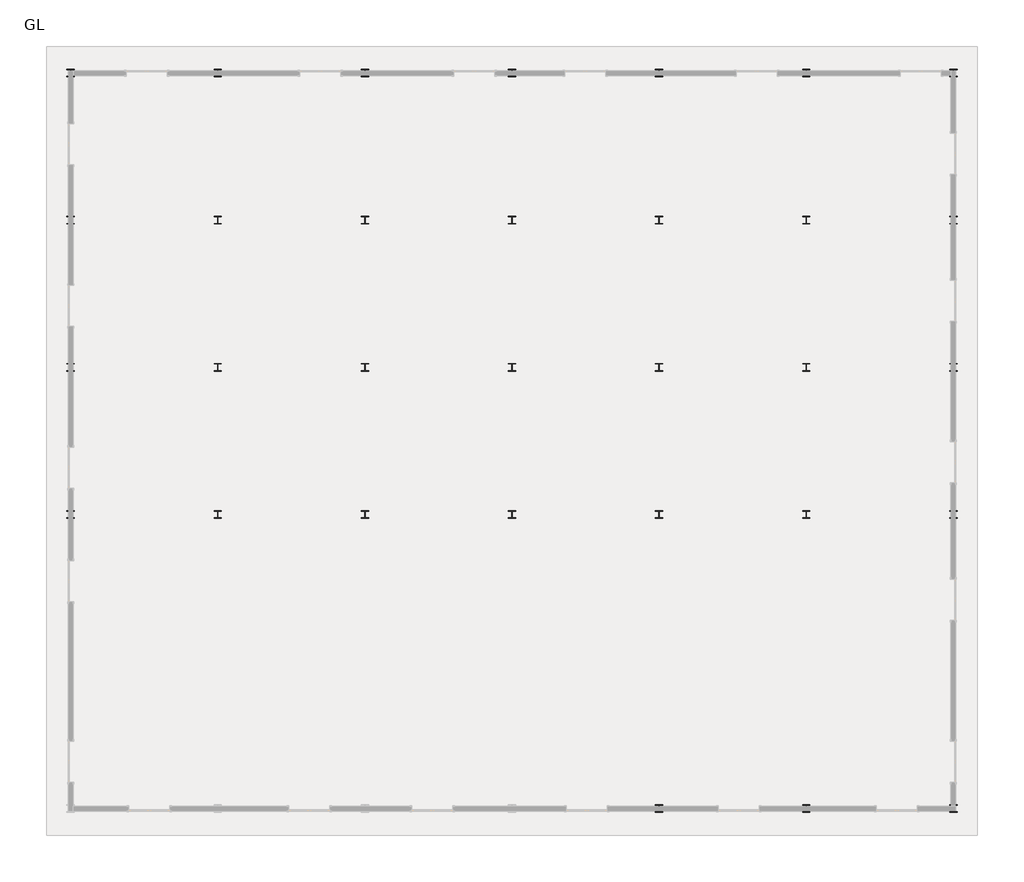
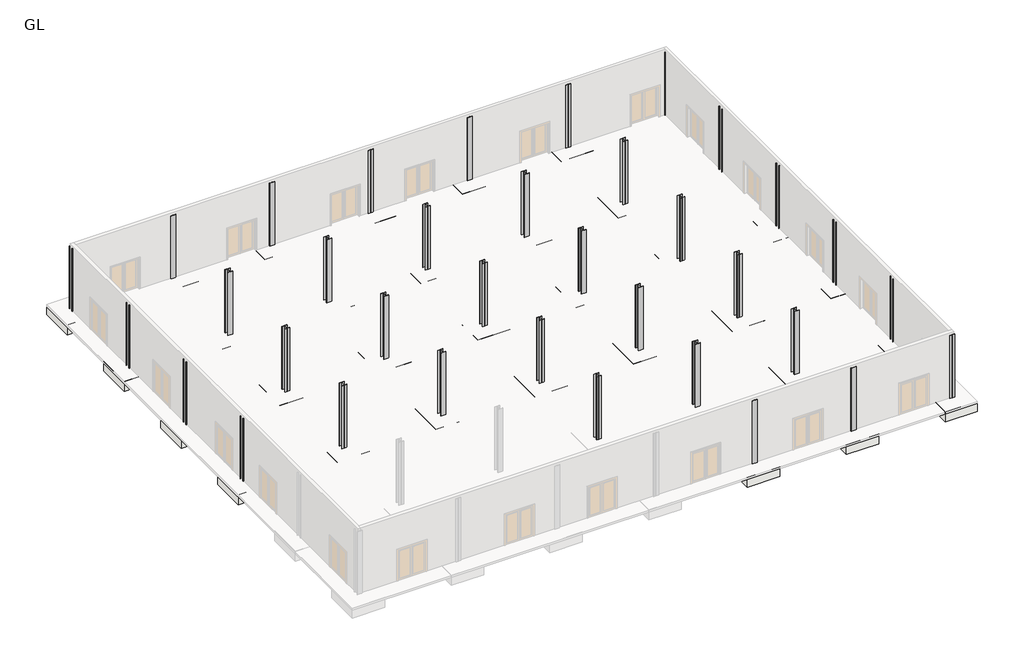
# One storey, part 2 of 2: 35 columns, 34 slabs.
"""IFC4 building model written with IfcOpenShell, lengths in millimetres."""

from ifc_helpers import new_model, si_unit, origin, place, context, project, spatial, transform, mapped, element, save
from components import uc_universal_columns_column_uc305x305x97_28816581, m_footing_rectangular_2200_x_2000_x_650mm_2_4a7b59ae

model = new_model("IFC4")

# Units and contexts
model_context = context("Model", 3, world=origin())
ifc_project = project(units=[si_unit("LENGTHUNIT", "METRE", prefix="MILLI")], contexts=[model_context])

# Site, building, storey
site = spatial("IfcSite", under=ifc_project)
building = spatial("IfcBuilding", under=site)
storey = spatial("IfcBuildingStorey", under=building, Name="GL", Elevation=-1812.3304639)

# Columns
placement = place(None, origin())
uc_universal_columns_column_uc305x305x97_shape = uc_universal_columns_column_uc305x305x97_28816581(model_context)
element("IfcColumn", 1, ObjectType="UC-Universal Columns-Column : UC305x305x97", at=placement, inside=storey, context=model_context, shape_type="MappedRepresentation", body=[
    mapped(uc_universal_columns_column_uc305x305x97_shape, transform((-18630.5493858, 24288.2691735, 0.0), x_axis=(1.0, 0.0, 0.0), y_axis=(0.0, 1.0, 0.0), z_axis=(0.0, 0.0, 1.0))),
])
element("IfcColumn", 2, ObjectType="UC-Universal Columns-Column : UC305x305x97", at=placement, inside=storey, context=model_context, shape_type="MappedRepresentation", body=[
    mapped(uc_universal_columns_column_uc305x305x97_shape, transform((5753.4506142, -6191.7308265, 0.0), x_axis=(1.0, 0.0, 0.0), y_axis=(0.0, 1.0, 0.0), z_axis=(0.0, 0.0, 1.0))),
])
element("IfcColumn", 3, ObjectType="UC-Universal Columns-Column : UC305x305x97", at=placement, inside=storey, context=model_context, shape_type="MappedRepresentation", body=[
    mapped(uc_universal_columns_column_uc305x305x97_shape, transform((11849.4506142, -6191.7308265, 0.0), x_axis=(1.0, 0.0, 0.0), y_axis=(0.0, 1.0, 0.0), z_axis=(0.0, 0.0, 1.0))),
])
element("IfcColumn", 4, ObjectType="UC-Universal Columns-Column : UC305x305x97", at=placement, inside=storey, context=model_context, shape_type="MappedRepresentation", body=[
    mapped(uc_universal_columns_column_uc305x305x97_shape, transform((17945.4506142, -6191.7308265, 0.0), x_axis=(1.0, 0.0, 0.0), y_axis=(0.0, 1.0, 0.0), z_axis=(0.0, 0.0, 1.0))),
])
element("IfcColumn", 5, ObjectType="UC-Universal Columns-Column : UC305x305x97", at=placement, inside=storey, context=model_context, shape_type="MappedRepresentation", body=[
    mapped(uc_universal_columns_column_uc305x305x97_shape, transform((-342.5493858, -95.7308265, 0.0), x_axis=(1.0, 0.0, 0.0), y_axis=(0.0, 1.0, 0.0), z_axis=(0.0, 0.0, 1.0))),
])
element("IfcColumn", 6, ObjectType="UC-Universal Columns-Column : UC305x305x97", at=placement, inside=storey, context=model_context, shape_type="MappedRepresentation", body=[
    mapped(uc_universal_columns_column_uc305x305x97_shape, transform((5753.4506142, -95.7308265, 0.0), x_axis=(1.0, 0.0, 0.0), y_axis=(0.0, 1.0, 0.0), z_axis=(0.0, 0.0, 1.0))),
])
element("IfcColumn", 7, ObjectType="UC-Universal Columns-Column : UC305x305x97", at=placement, inside=storey, context=model_context, shape_type="MappedRepresentation", body=[
    mapped(uc_universal_columns_column_uc305x305x97_shape, transform((11849.4506142, -95.7308265, 0.0), x_axis=(1.0, 0.0, 0.0), y_axis=(0.0, 1.0, 0.0), z_axis=(0.0, 0.0, 1.0))),
])
element("IfcColumn", 8, ObjectType="UC-Universal Columns-Column : UC305x305x97", at=placement, inside=storey, context=model_context, shape_type="MappedRepresentation", body=[
    mapped(uc_universal_columns_column_uc305x305x97_shape, transform((17945.4506142, -95.7308265, 0.0), x_axis=(1.0, 0.0, 0.0), y_axis=(0.0, 1.0, 0.0), z_axis=(0.0, 0.0, 1.0))),
])
element("IfcColumn", 9, ObjectType="UC-Universal Columns-Column : UC305x305x97", at=placement, inside=storey, context=model_context, shape_type="MappedRepresentation", body=[
    mapped(uc_universal_columns_column_uc305x305x97_shape, transform((-18630.5493858, 6000.2691735, 0.0), x_axis=(1.0, 0.0, 0.0), y_axis=(0.0, 1.0, 0.0), z_axis=(0.0, 0.0, 1.0))),
])
element("IfcColumn", 10, ObjectType="UC-Universal Columns-Column : UC305x305x97", at=placement, inside=storey, context=model_context, shape_type="MappedRepresentation", body=[
    mapped(uc_universal_columns_column_uc305x305x97_shape, transform((-12534.5493858, 6000.2691735, 0.0), x_axis=(1.0, 0.0, 0.0), y_axis=(0.0, 1.0, 0.0), z_axis=(0.0, 0.0, 1.0))),
])
element("IfcColumn", 11, ObjectType="UC-Universal Columns-Column : UC305x305x97", at=placement, inside=storey, context=model_context, shape_type="MappedRepresentation", body=[
    mapped(uc_universal_columns_column_uc305x305x97_shape, transform((-6438.5493858, 6000.2691735, 0.0), x_axis=(1.0, 0.0, 0.0), y_axis=(0.0, 1.0, 0.0), z_axis=(0.0, 0.0, 1.0))),
])
element("IfcColumn", 12, ObjectType="UC-Universal Columns-Column : UC305x305x97", at=placement, inside=storey, context=model_context, shape_type="MappedRepresentation", body=[
    mapped(uc_universal_columns_column_uc305x305x97_shape, transform((-342.5493858, 6000.2691735, 0.0), x_axis=(1.0, 0.0, 0.0), y_axis=(0.0, 1.0, 0.0), z_axis=(0.0, 0.0, 1.0))),
])
element("IfcColumn", 13, ObjectType="UC-Universal Columns-Column : UC305x305x97", at=placement, inside=storey, context=model_context, shape_type="MappedRepresentation", body=[
    mapped(uc_universal_columns_column_uc305x305x97_shape, transform((5753.4506142, 6000.2691735, 0.0), x_axis=(1.0, 0.0, 0.0), y_axis=(0.0, 1.0, 0.0), z_axis=(0.0, 0.0, 1.0))),
])
element("IfcColumn", 14, ObjectType="UC-Universal Columns-Column : UC305x305x97", at=placement, inside=storey, context=model_context, shape_type="MappedRepresentation", body=[
    mapped(uc_universal_columns_column_uc305x305x97_shape, transform((11849.4506142, 6000.2691735, 0.0), x_axis=(1.0, 0.0, 0.0), y_axis=(0.0, 1.0, 0.0), z_axis=(0.0, 0.0, 1.0))),
])
element("IfcColumn", 15, ObjectType="UC-Universal Columns-Column : UC305x305x97", at=placement, inside=storey, context=model_context, shape_type="MappedRepresentation", body=[
    mapped(uc_universal_columns_column_uc305x305x97_shape, transform((17945.4506142, 6000.2691735, 0.0), x_axis=(1.0, 0.0, 0.0), y_axis=(0.0, 1.0, 0.0), z_axis=(0.0, 0.0, 1.0))),
])
element("IfcColumn", 16, ObjectType="UC-Universal Columns-Column : UC305x305x97", at=placement, inside=storey, context=model_context, shape_type="MappedRepresentation", body=[
    mapped(uc_universal_columns_column_uc305x305x97_shape, transform((-18630.5493858, 12096.2691735, 0.0), x_axis=(1.0, 0.0, 0.0), y_axis=(0.0, 1.0, 0.0), z_axis=(0.0, 0.0, 1.0))),
])
element("IfcColumn", 17, ObjectType="UC-Universal Columns-Column : UC305x305x97", at=placement, inside=storey, context=model_context, shape_type="MappedRepresentation", body=[
    mapped(uc_universal_columns_column_uc305x305x97_shape, transform((-12534.5493858, 12096.2691735, 0.0), x_axis=(1.0, 0.0, 0.0), y_axis=(0.0, 1.0, 0.0), z_axis=(0.0, 0.0, 1.0))),
])
element("IfcColumn", 18, ObjectType="UC-Universal Columns-Column : UC305x305x97", at=placement, inside=storey, context=model_context, shape_type="MappedRepresentation", body=[
    mapped(uc_universal_columns_column_uc305x305x97_shape, transform((-6438.5493858, 12096.2691735, 0.0), x_axis=(1.0, 0.0, 0.0), y_axis=(0.0, 1.0, 0.0), z_axis=(0.0, 0.0, 1.0))),
])
element("IfcColumn", 19, ObjectType="UC-Universal Columns-Column : UC305x305x97", at=placement, inside=storey, context=model_context, shape_type="MappedRepresentation", body=[
    mapped(uc_universal_columns_column_uc305x305x97_shape, transform((-342.5493858, 12096.2691735, 0.0), x_axis=(1.0, 0.0, 0.0), y_axis=(0.0, 1.0, 0.0), z_axis=(0.0, 0.0, 1.0))),
])
element("IfcColumn", 20, ObjectType="UC-Universal Columns-Column : UC305x305x97", at=placement, inside=storey, context=model_context, shape_type="MappedRepresentation", body=[
    mapped(uc_universal_columns_column_uc305x305x97_shape, transform((5753.4506142, 12096.2691735, 0.0), x_axis=(1.0, 0.0, 0.0), y_axis=(0.0, 1.0, 0.0), z_axis=(0.0, 0.0, 1.0))),
])
element("IfcColumn", 21, ObjectType="UC-Universal Columns-Column : UC305x305x97", at=placement, inside=storey, context=model_context, shape_type="MappedRepresentation", body=[
    mapped(uc_universal_columns_column_uc305x305x97_shape, transform((11849.4506142, 12096.2691735, 0.0), x_axis=(1.0, 0.0, 0.0), y_axis=(0.0, 1.0, 0.0), z_axis=(0.0, 0.0, 1.0))),
])
element("IfcColumn", 22, ObjectType="UC-Universal Columns-Column : UC305x305x97", at=placement, inside=storey, context=model_context, shape_type="MappedRepresentation", body=[
    mapped(uc_universal_columns_column_uc305x305x97_shape, transform((17945.4506142, 12096.2691735, 0.0), x_axis=(1.0, 0.0, 0.0), y_axis=(0.0, 1.0, 0.0), z_axis=(0.0, 0.0, 1.0))),
])
element("IfcColumn", 23, ObjectType="UC-Universal Columns-Column : UC305x305x97", at=placement, inside=storey, context=model_context, shape_type="MappedRepresentation", body=[
    mapped(uc_universal_columns_column_uc305x305x97_shape, transform((-18630.5493858, 18192.2691735, 0.0), x_axis=(1.0, 0.0, 0.0), y_axis=(0.0, 1.0, 0.0), z_axis=(0.0, 0.0, 1.0))),
])
element("IfcColumn", 24, ObjectType="UC-Universal Columns-Column : UC305x305x97", at=placement, inside=storey, context=model_context, shape_type="MappedRepresentation", body=[
    mapped(uc_universal_columns_column_uc305x305x97_shape, transform((-12534.5493858, 18192.2691735, 0.0), x_axis=(1.0, 0.0, 0.0), y_axis=(0.0, 1.0, 0.0), z_axis=(0.0, 0.0, 1.0))),
])
element("IfcColumn", 25, ObjectType="UC-Universal Columns-Column : UC305x305x97", at=placement, inside=storey, context=model_context, shape_type="MappedRepresentation", body=[
    mapped(uc_universal_columns_column_uc305x305x97_shape, transform((-6438.5493858, 18192.2691735, 0.0), x_axis=(1.0, 0.0, 0.0), y_axis=(0.0, 1.0, 0.0), z_axis=(0.0, 0.0, 1.0))),
])
element("IfcColumn", 26, ObjectType="UC-Universal Columns-Column : UC305x305x97", at=placement, inside=storey, context=model_context, shape_type="MappedRepresentation", body=[
    mapped(uc_universal_columns_column_uc305x305x97_shape, transform((-342.5493858, 18192.2691735, 0.0), x_axis=(1.0, 0.0, 0.0), y_axis=(0.0, 1.0, 0.0), z_axis=(0.0, 0.0, 1.0))),
])
element("IfcColumn", 27, ObjectType="UC-Universal Columns-Column : UC305x305x97", at=placement, inside=storey, context=model_context, shape_type="MappedRepresentation", body=[
    mapped(uc_universal_columns_column_uc305x305x97_shape, transform((5753.4506142, 18192.2691735, 0.0), x_axis=(1.0, 0.0, 0.0), y_axis=(0.0, 1.0, 0.0), z_axis=(0.0, 0.0, 1.0))),
])
element("IfcColumn", 28, ObjectType="UC-Universal Columns-Column : UC305x305x97", at=placement, inside=storey, context=model_context, shape_type="MappedRepresentation", body=[
    mapped(uc_universal_columns_column_uc305x305x97_shape, transform((11849.4506142, 18192.2691735, 0.0), x_axis=(1.0, 0.0, 0.0), y_axis=(0.0, 1.0, 0.0), z_axis=(0.0, 0.0, 1.0))),
])
element("IfcColumn", 29, ObjectType="UC-Universal Columns-Column : UC305x305x97", at=placement, inside=storey, context=model_context, shape_type="MappedRepresentation", body=[
    mapped(uc_universal_columns_column_uc305x305x97_shape, transform((17945.4506142, 18192.2691735, 0.0), x_axis=(1.0, 0.0, 0.0), y_axis=(0.0, 1.0, 0.0), z_axis=(0.0, 0.0, 1.0))),
])
element("IfcColumn", 30, ObjectType="UC-Universal Columns-Column : UC305x305x97", at=placement, inside=storey, context=model_context, shape_type="MappedRepresentation", body=[
    mapped(uc_universal_columns_column_uc305x305x97_shape, transform((-12534.5493858, 24288.2691735, 0.0), x_axis=(1.0, 0.0, 0.0), y_axis=(0.0, 1.0, 0.0), z_axis=(0.0, 0.0, 1.0))),
])
element("IfcColumn", 31, ObjectType="UC-Universal Columns-Column : UC305x305x97", at=placement, inside=storey, context=model_context, shape_type="MappedRepresentation", body=[
    mapped(uc_universal_columns_column_uc305x305x97_shape, transform((-6438.5493858, 24288.2691735, 0.0), x_axis=(1.0, 0.0, 0.0), y_axis=(0.0, 1.0, 0.0), z_axis=(0.0, 0.0, 1.0))),
])
element("IfcColumn", 32, ObjectType="UC-Universal Columns-Column : UC305x305x97", at=placement, inside=storey, context=model_context, shape_type="MappedRepresentation", body=[
    mapped(uc_universal_columns_column_uc305x305x97_shape, transform((-342.5493858, 24288.2691735, 0.0), x_axis=(1.0, 0.0, 0.0), y_axis=(0.0, 1.0, 0.0), z_axis=(0.0, 0.0, 1.0))),
])
element("IfcColumn", 33, ObjectType="UC-Universal Columns-Column : UC305x305x97", at=placement, inside=storey, context=model_context, shape_type="MappedRepresentation", body=[
    mapped(uc_universal_columns_column_uc305x305x97_shape, transform((5753.4506142, 24288.2691735, 0.0), x_axis=(1.0, 0.0, 0.0), y_axis=(0.0, 1.0, 0.0), z_axis=(0.0, 0.0, 1.0))),
])
element("IfcColumn", 34, ObjectType="UC-Universal Columns-Column : UC305x305x97", at=placement, inside=storey, context=model_context, shape_type="MappedRepresentation", body=[
    mapped(uc_universal_columns_column_uc305x305x97_shape, transform((11849.4506142, 24288.2691735, 0.0), x_axis=(1.0, 0.0, 0.0), y_axis=(0.0, 1.0, 0.0), z_axis=(0.0, 0.0, 1.0))),
])
element("IfcColumn", 35, ObjectType="UC-Universal Columns-Column : UC305x305x97", at=placement, inside=storey, context=model_context, shape_type="MappedRepresentation", body=[
    mapped(uc_universal_columns_column_uc305x305x97_shape, transform((17945.4506142, 24288.2691735, 0.0), x_axis=(1.0, 0.0, 0.0), y_axis=(0.0, 1.0, 0.0), z_axis=(0.0, 0.0, 1.0))),
])

# Slabs
m_footing_rectangular_2200_x_2000_x_650mm_2_shape = m_footing_rectangular_2200_x_2000_x_650mm_2_4a7b59ae(model_context)
element("IfcSlab", 36, ObjectType="M_Footing-Rectangular : 2200 x 2000 x 650mm 2", at=placement, inside=storey, context=model_context, shape_type="MappedRepresentation", body=[
    mapped(m_footing_rectangular_2200_x_2000_x_650mm_2_shape, transform((-18630.5493858, 24288.2691735, -1812.3304639), x_axis=(1.0, 0.0, 0.0), y_axis=(0.0, 1.0, 0.0), z_axis=(0.0, 0.0, 1.0))),
])
element("IfcSlab", 37, ObjectType="M_Footing-Rectangular : 2200 x 2000 x 650mm 2", at=placement, inside=storey, context=model_context, shape_type="MappedRepresentation", body=[
    mapped(m_footing_rectangular_2200_x_2000_x_650mm_2_shape, transform((5753.4506142, -6191.7308265, -1812.3304639), x_axis=(1.0, 0.0, 0.0), y_axis=(0.0, 1.0, 0.0), z_axis=(0.0, 0.0, 1.0))),
])
element("IfcSlab", 38, ObjectType="M_Footing-Rectangular : 2200 x 2000 x 650mm 2", at=placement, inside=storey, context=model_context, shape_type="MappedRepresentation", body=[
    mapped(m_footing_rectangular_2200_x_2000_x_650mm_2_shape, transform((11849.4506142, -6191.7308265, -1812.3304639), x_axis=(1.0, 0.0, 0.0), y_axis=(0.0, 1.0, 0.0), z_axis=(0.0, 0.0, 1.0))),
])
element("IfcSlab", 39, ObjectType="M_Footing-Rectangular : 2200 x 2000 x 650mm 2", at=placement, inside=storey, context=model_context, shape_type="MappedRepresentation", body=[
    mapped(m_footing_rectangular_2200_x_2000_x_650mm_2_shape, transform((17945.4506142, -6191.7308265, -1812.3304639), x_axis=(1.0, 0.0, 0.0), y_axis=(0.0, 1.0, 0.0), z_axis=(0.0, 0.0, 1.0))),
])
element("IfcSlab", 40, ObjectType="M_Footing-Rectangular : 2200 x 2000 x 650mm 2", at=placement, inside=storey, context=model_context, shape_type="MappedRepresentation", body=[
    mapped(m_footing_rectangular_2200_x_2000_x_650mm_2_shape, transform((5753.4506142, -95.7308265, -1812.3304639), x_axis=(1.0, 0.0, 0.0), y_axis=(0.0, 1.0, 0.0), z_axis=(0.0, 0.0, 1.0))),
])
element("IfcSlab", 41, ObjectType="M_Footing-Rectangular : 2200 x 2000 x 650mm 2", at=placement, inside=storey, context=model_context, shape_type="MappedRepresentation", body=[
    mapped(m_footing_rectangular_2200_x_2000_x_650mm_2_shape, transform((11849.4506142, -95.7308265, -1812.3304639), x_axis=(1.0, 0.0, 0.0), y_axis=(0.0, 1.0, 0.0), z_axis=(0.0, 0.0, 1.0))),
])
element("IfcSlab", 42, ObjectType="M_Footing-Rectangular : 2200 x 2000 x 650mm 2", at=placement, inside=storey, context=model_context, shape_type="MappedRepresentation", body=[
    mapped(m_footing_rectangular_2200_x_2000_x_650mm_2_shape, transform((17945.4506142, -95.7308265, -1812.3304639), x_axis=(1.0, 0.0, 0.0), y_axis=(0.0, 1.0, 0.0), z_axis=(0.0, 0.0, 1.0))),
])
element("IfcSlab", 43, ObjectType="M_Footing-Rectangular : 2200 x 2000 x 650mm 2", at=placement, inside=storey, context=model_context, shape_type="MappedRepresentation", body=[
    mapped(m_footing_rectangular_2200_x_2000_x_650mm_2_shape, transform((-18630.5493858, 6000.2691735, -1812.3304639), x_axis=(1.0, 0.0, 0.0), y_axis=(0.0, 1.0, 0.0), z_axis=(0.0, 0.0, 1.0))),
])
element("IfcSlab", 44, ObjectType="M_Footing-Rectangular : 2200 x 2000 x 650mm 2", at=placement, inside=storey, context=model_context, shape_type="MappedRepresentation", body=[
    mapped(m_footing_rectangular_2200_x_2000_x_650mm_2_shape, transform((-12534.5493858, 6000.2691735, -1812.3304639), x_axis=(1.0, 0.0, 0.0), y_axis=(0.0, 1.0, 0.0), z_axis=(0.0, 0.0, 1.0))),
])
element("IfcSlab", 45, ObjectType="M_Footing-Rectangular : 2200 x 2000 x 650mm 2", at=placement, inside=storey, context=model_context, shape_type="MappedRepresentation", body=[
    mapped(m_footing_rectangular_2200_x_2000_x_650mm_2_shape, transform((-6438.5493858, 6000.2691735, -1812.3304639), x_axis=(1.0, 0.0, 0.0), y_axis=(0.0, 1.0, 0.0), z_axis=(0.0, 0.0, 1.0))),
])
element("IfcSlab", 46, ObjectType="M_Footing-Rectangular : 2200 x 2000 x 650mm 2", at=placement, inside=storey, context=model_context, shape_type="MappedRepresentation", body=[
    mapped(m_footing_rectangular_2200_x_2000_x_650mm_2_shape, transform((-342.5493858, 6000.2691735, -1812.3304639), x_axis=(1.0, 0.0, 0.0), y_axis=(0.0, 1.0, 0.0), z_axis=(0.0, 0.0, 1.0))),
])
element("IfcSlab", 47, ObjectType="M_Footing-Rectangular : 2200 x 2000 x 650mm 2", at=placement, inside=storey, context=model_context, shape_type="MappedRepresentation", body=[
    mapped(m_footing_rectangular_2200_x_2000_x_650mm_2_shape, transform((5753.4506142, 6000.2691735, -1812.3304639), x_axis=(1.0, 0.0, 0.0), y_axis=(0.0, 1.0, 0.0), z_axis=(0.0, 0.0, 1.0))),
])
element("IfcSlab", 48, ObjectType="M_Footing-Rectangular : 2200 x 2000 x 650mm 2", at=placement, inside=storey, context=model_context, shape_type="MappedRepresentation", body=[
    mapped(m_footing_rectangular_2200_x_2000_x_650mm_2_shape, transform((11849.4506142, 6000.2691735, -1812.3304639), x_axis=(1.0, 0.0, 0.0), y_axis=(0.0, 1.0, 0.0), z_axis=(0.0, 0.0, 1.0))),
])
element("IfcSlab", 49, ObjectType="M_Footing-Rectangular : 2200 x 2000 x 650mm 2", at=placement, inside=storey, context=model_context, shape_type="MappedRepresentation", body=[
    mapped(m_footing_rectangular_2200_x_2000_x_650mm_2_shape, transform((17945.4506142, 6000.2691735, -1812.3304639), x_axis=(1.0, 0.0, 0.0), y_axis=(0.0, 1.0, 0.0), z_axis=(0.0, 0.0, 1.0))),
])
element("IfcSlab", 50, ObjectType="M_Footing-Rectangular : 2200 x 2000 x 650mm 2", at=placement, inside=storey, context=model_context, shape_type="MappedRepresentation", body=[
    mapped(m_footing_rectangular_2200_x_2000_x_650mm_2_shape, transform((-18630.5493858, 12096.2691735, -1812.3304639), x_axis=(1.0, 0.0, 0.0), y_axis=(0.0, 1.0, 0.0), z_axis=(0.0, 0.0, 1.0))),
])
element("IfcSlab", 51, ObjectType="M_Footing-Rectangular : 2200 x 2000 x 650mm 2", at=placement, inside=storey, context=model_context, shape_type="MappedRepresentation", body=[
    mapped(m_footing_rectangular_2200_x_2000_x_650mm_2_shape, transform((-12534.5493858, 12096.2691735, -1812.3304639), x_axis=(1.0, 0.0, 0.0), y_axis=(0.0, 1.0, 0.0), z_axis=(0.0, 0.0, 1.0))),
])
element("IfcSlab", 52, ObjectType="M_Footing-Rectangular : 2200 x 2000 x 650mm 2", at=placement, inside=storey, context=model_context, shape_type="MappedRepresentation", body=[
    mapped(m_footing_rectangular_2200_x_2000_x_650mm_2_shape, transform((-6438.5493858, 12096.2691735, -1812.3304639), x_axis=(1.0, 0.0, 0.0), y_axis=(0.0, 1.0, 0.0), z_axis=(0.0, 0.0, 1.0))),
])
element("IfcSlab", 53, ObjectType="M_Footing-Rectangular : 2200 x 2000 x 650mm 2", at=placement, inside=storey, context=model_context, shape_type="MappedRepresentation", body=[
    mapped(m_footing_rectangular_2200_x_2000_x_650mm_2_shape, transform((-342.5493858, 12096.2691735, -1812.3304639), x_axis=(1.0, 0.0, 0.0), y_axis=(0.0, 1.0, 0.0), z_axis=(0.0, 0.0, 1.0))),
])
element("IfcSlab", 54, ObjectType="M_Footing-Rectangular : 2200 x 2000 x 650mm 2", at=placement, inside=storey, context=model_context, shape_type="MappedRepresentation", body=[
    mapped(m_footing_rectangular_2200_x_2000_x_650mm_2_shape, transform((5753.4506142, 12096.2691735, -1812.3304639), x_axis=(1.0, 0.0, 0.0), y_axis=(0.0, 1.0, 0.0), z_axis=(0.0, 0.0, 1.0))),
])
element("IfcSlab", 55, ObjectType="M_Footing-Rectangular : 2200 x 2000 x 650mm 2", at=placement, inside=storey, context=model_context, shape_type="MappedRepresentation", body=[
    mapped(m_footing_rectangular_2200_x_2000_x_650mm_2_shape, transform((11849.4506142, 12096.2691735, -1812.3304639), x_axis=(1.0, 0.0, 0.0), y_axis=(0.0, 1.0, 0.0), z_axis=(0.0, 0.0, 1.0))),
])
element("IfcSlab", 56, ObjectType="M_Footing-Rectangular : 2200 x 2000 x 650mm 2", at=placement, inside=storey, context=model_context, shape_type="MappedRepresentation", body=[
    mapped(m_footing_rectangular_2200_x_2000_x_650mm_2_shape, transform((17945.4506142, 12096.2691735, -1812.3304639), x_axis=(1.0, 0.0, 0.0), y_axis=(0.0, 1.0, 0.0), z_axis=(0.0, 0.0, 1.0))),
])
element("IfcSlab", 57, ObjectType="M_Footing-Rectangular : 2200 x 2000 x 650mm 2", at=placement, inside=storey, context=model_context, shape_type="MappedRepresentation", body=[
    mapped(m_footing_rectangular_2200_x_2000_x_650mm_2_shape, transform((-18630.5493858, 18192.2691735, -1812.3304639), x_axis=(1.0, 0.0, 0.0), y_axis=(0.0, 1.0, 0.0), z_axis=(0.0, 0.0, 1.0))),
])
element("IfcSlab", 58, ObjectType="M_Footing-Rectangular : 2200 x 2000 x 650mm 2", at=placement, inside=storey, context=model_context, shape_type="MappedRepresentation", body=[
    mapped(m_footing_rectangular_2200_x_2000_x_650mm_2_shape, transform((-12534.5493858, 18192.2691735, -1812.3304639), x_axis=(1.0, 0.0, 0.0), y_axis=(0.0, 1.0, 0.0), z_axis=(0.0, 0.0, 1.0))),
])
element("IfcSlab", 59, ObjectType="M_Footing-Rectangular : 2200 x 2000 x 650mm 2", at=placement, inside=storey, context=model_context, shape_type="MappedRepresentation", body=[
    mapped(m_footing_rectangular_2200_x_2000_x_650mm_2_shape, transform((-6438.5493858, 18192.2691735, -1812.3304639), x_axis=(1.0, 0.0, 0.0), y_axis=(0.0, 1.0, 0.0), z_axis=(0.0, 0.0, 1.0))),
])
element("IfcSlab", 60, ObjectType="M_Footing-Rectangular : 2200 x 2000 x 650mm 2", at=placement, inside=storey, context=model_context, shape_type="MappedRepresentation", body=[
    mapped(m_footing_rectangular_2200_x_2000_x_650mm_2_shape, transform((-342.5493858, 18192.2691735, -1812.3304639), x_axis=(1.0, 0.0, 0.0), y_axis=(0.0, 1.0, 0.0), z_axis=(0.0, 0.0, 1.0))),
])
element("IfcSlab", 61, ObjectType="M_Footing-Rectangular : 2200 x 2000 x 650mm 2", at=placement, inside=storey, context=model_context, shape_type="MappedRepresentation", body=[
    mapped(m_footing_rectangular_2200_x_2000_x_650mm_2_shape, transform((5753.4506142, 18192.2691735, -1812.3304639), x_axis=(1.0, 0.0, 0.0), y_axis=(0.0, 1.0, 0.0), z_axis=(0.0, 0.0, 1.0))),
])
element("IfcSlab", 62, ObjectType="M_Footing-Rectangular : 2200 x 2000 x 650mm 2", at=placement, inside=storey, context=model_context, shape_type="MappedRepresentation", body=[
    mapped(m_footing_rectangular_2200_x_2000_x_650mm_2_shape, transform((11849.4506142, 18192.2691735, -1812.3304639), x_axis=(1.0, 0.0, 0.0), y_axis=(0.0, 1.0, 0.0), z_axis=(0.0, 0.0, 1.0))),
])
element("IfcSlab", 63, ObjectType="M_Footing-Rectangular : 2200 x 2000 x 650mm 2", at=placement, inside=storey, context=model_context, shape_type="MappedRepresentation", body=[
    mapped(m_footing_rectangular_2200_x_2000_x_650mm_2_shape, transform((17945.4506142, 18192.2691735, -1812.3304639), x_axis=(1.0, 0.0, 0.0), y_axis=(0.0, 1.0, 0.0), z_axis=(0.0, 0.0, 1.0))),
])
element("IfcSlab", 64, ObjectType="M_Footing-Rectangular : 2200 x 2000 x 650mm 2", at=placement, inside=storey, context=model_context, shape_type="MappedRepresentation", body=[
    mapped(m_footing_rectangular_2200_x_2000_x_650mm_2_shape, transform((-12534.5493858, 24288.2691735, -1812.3304639), x_axis=(1.0, 0.0, 0.0), y_axis=(0.0, 1.0, 0.0), z_axis=(0.0, 0.0, 1.0))),
])
element("IfcSlab", 65, ObjectType="M_Footing-Rectangular : 2200 x 2000 x 650mm 2", at=placement, inside=storey, context=model_context, shape_type="MappedRepresentation", body=[
    mapped(m_footing_rectangular_2200_x_2000_x_650mm_2_shape, transform((-6438.5493858, 24288.2691735, -1812.3304639), x_axis=(1.0, 0.0, 0.0), y_axis=(0.0, 1.0, 0.0), z_axis=(0.0, 0.0, 1.0))),
])
element("IfcSlab", 66, ObjectType="M_Footing-Rectangular : 2200 x 2000 x 650mm 2", at=placement, inside=storey, context=model_context, shape_type="MappedRepresentation", body=[
    mapped(m_footing_rectangular_2200_x_2000_x_650mm_2_shape, transform((-342.5493858, 24288.2691735, -1812.3304639), x_axis=(1.0, 0.0, 0.0), y_axis=(0.0, 1.0, 0.0), z_axis=(0.0, 0.0, 1.0))),
])
element("IfcSlab", 67, ObjectType="M_Footing-Rectangular : 2200 x 2000 x 650mm 2", at=placement, inside=storey, context=model_context, shape_type="MappedRepresentation", body=[
    mapped(m_footing_rectangular_2200_x_2000_x_650mm_2_shape, transform((5753.4506142, 24288.2691735, -1812.3304639), x_axis=(1.0, 0.0, 0.0), y_axis=(0.0, 1.0, 0.0), z_axis=(0.0, 0.0, 1.0))),
])
element("IfcSlab", 68, ObjectType="M_Footing-Rectangular : 2200 x 2000 x 650mm 2", at=placement, inside=storey, context=model_context, shape_type="MappedRepresentation", body=[
    mapped(m_footing_rectangular_2200_x_2000_x_650mm_2_shape, transform((11849.4506142, 24288.2691735, -1812.3304639), x_axis=(1.0, 0.0, 0.0), y_axis=(0.0, 1.0, 0.0), z_axis=(0.0, 0.0, 1.0))),
])
element("IfcSlab", 69, ObjectType="M_Footing-Rectangular : 2200 x 2000 x 650mm 2", at=placement, inside=storey, context=model_context, shape_type="MappedRepresentation", body=[
    mapped(m_footing_rectangular_2200_x_2000_x_650mm_2_shape, transform((17945.4506142, 24288.2691735, -1812.3304639), x_axis=(1.0, 0.0, 0.0), y_axis=(0.0, 1.0, 0.0), z_axis=(0.0, 0.0, 1.0))),
])

save(model, "model.ifc")

# Revit data of these elements
# Type "UC-Universal Columns-Column : UC305x305x97"
#   Section Name Key = "UC305x305x97"
#   Width = 30.53 cm
#   Web Thickness = 0.99 cm
#   Web Fillet = 1.52 cm
#   Warping Constant = 1560000.0 cm⁶
#   Torsional Moment of Inertia = 91.20 cm⁴
#   Section Area = 123.0 cm²
#   Plastic Modulus weak axis = 726.0 cm³
#   Plastic Modulus strong axis = 1592.0 cm³
#   Nominal Weight = 96.8996 kgf/m
#   Moment of Inertia weak axis = 7308.00 cm⁴
#   Moment of Inertia strong axis = 22249.00 cm⁴
#   Height = 30.79 cm
#   Flange Thickness = 1.54 cm
#   Elastic Modulus weak axis = 479.0 cm³
#   Elastic Modulus strong axis = 1445.0 cm³
#   Centroid Vertical = 15.395 cm
#   Centroid Horizontal = 15.265 cm
#   Bolt Spacing = 14.0 cm
#   Structural Material [instance default] = Metal - Steel 43-275
#   Type Comments = ""
#   Assembly Code = ""
# Type "M_Footing-Rectangular : 2200 x 2000 x 650mm 2"
#   Width = 2000 mm
#   Length = 2200 mm
#   Foundation Thickness = 650 mm
#   Structural Material [instance default] = Concrete, Cast-in-Place gray
#   Assembly Code = ""
# Elements 1, 2, 3, 4, 5, 6, 7, 8, 9, 10, 11, 12, 13, 14, 15, 16, 17, 18, 19, 20, 21, 22, 23, 24, 25, 26, 27, 28, 29, 30, 31, 32, 33, 34, 35 (IfcColumn, "UC-Universal Columns-Column : UC305x305x97")
#   Structural Material = Metal - Steel 43-275
#   Phase Created = New Construction
#   Materials on its faces: "Metal - Steel 43-275"
# Elements 36, 37, 38, 39, 40, 41, 42, 43, 44, 45, 46, 47, 48, 49, 50, 51, 52, 53, 54, 55, 56, 57, 58, 59, 60, 61, 62, 63, 64, 65, 66, 67, 68, 69 (IfcSlab, "M_Footing-Rectangular : 2200 x 2000 x 650mm 2")
#   Structural Material = Concrete, Cast-in-Place gray
#   Phase Created = New Construction
#   Materials on its faces: "Concrete, Cast-in-Place gray"
# Materials
#   "Metal - Steel 43-275": class "Metal", colour RGB 247 247 247, transparency 0, Cost = 0
#   "Concrete, Cast-in-Place gray": class "Concrete", colour RGB 192 192 192, transparency 0, Description = "Cast-in-place concrete", Cost = 0
